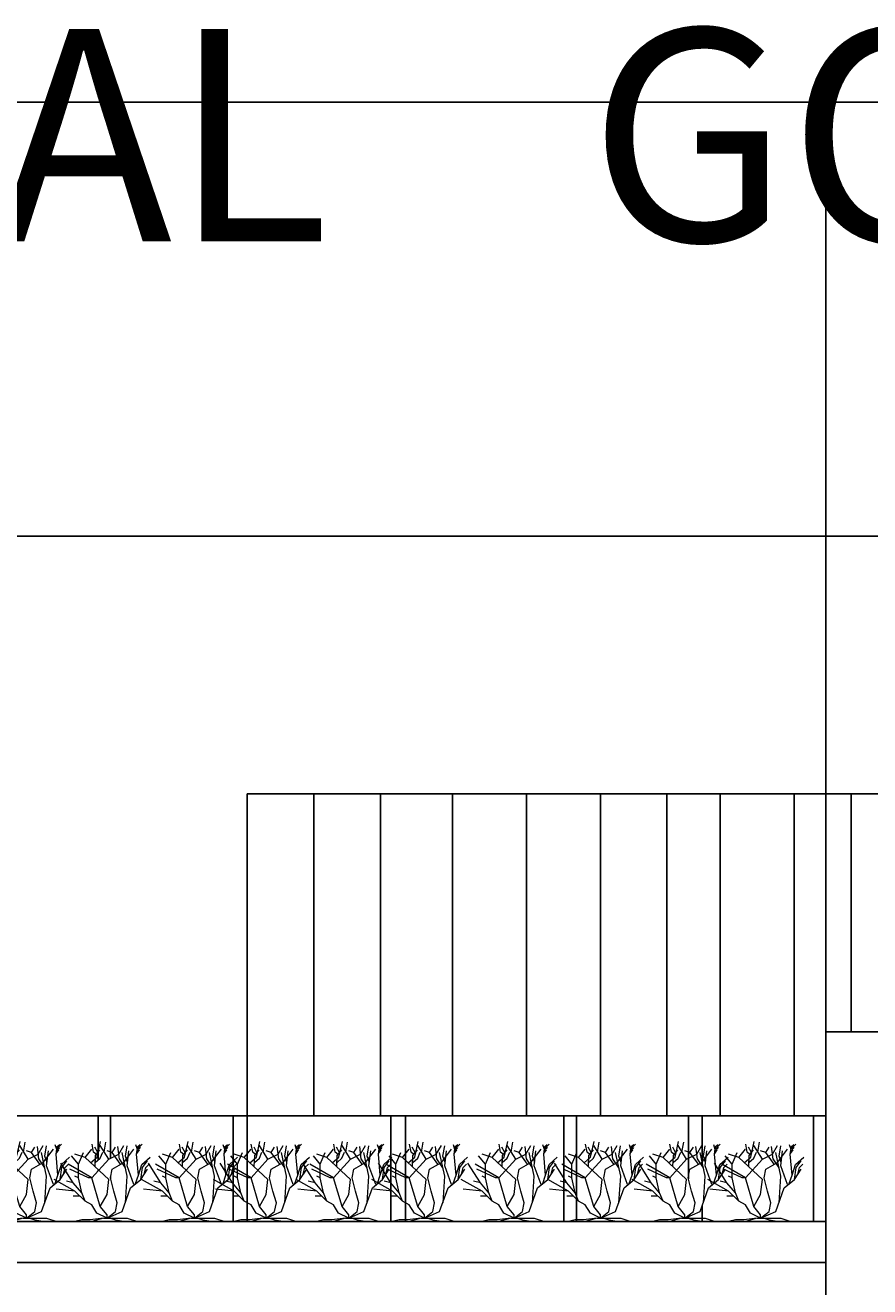
# Model space of a CAD drawing. Units: inches. Extents: x -117 to 121, y -77 to 40.
# Tile 17 of 45: x -45 to -23, y 7 to 40. Entities that reach past the tile are written whole.
import ezdxf

# ---------------------------------------------------------------- set-up
doc = ezdxf.new("R2010")
doc.units = ezdxf.units.IN
doc.header["$MEASUREMENT"] = 0
for name, color, linetype, lineweight in [('A-ANNO-DIMS', 2, 'Continuous', 18), ('A-ANNO-TEXT', 7, 'Continuous', 25), ('A-ELEV', 7, 'Continuous', 25), ('L-PLNT', 3, 'Continuous', 13)]:
    doc.layers.add(name, color=color, linetype=linetype, lineweight=lineweight)
doc.styles.get("Standard").update_dxf_attribs({"font": 'arial.ttf'})
doc.dimstyles.get("Standard").update_dxf_attribs({"dimtxt": 0.18, "dimasz": 0.18, "dimexe": 0.18, "dimexo": 0.0625, "dimgap": 0.09, "dimtad": 0, "dimtih": 1, "dimtoh": 1, "dimdec": 4, "dimzin": 0, "dimdsep": 46, "dimtxsty": 'Standard', "dimcen": 0.09, "dimadec": 0, "dimazin": 0, "dimtfac": 1, "dimtdec": 4, "dimtofl": 0, "dimtmove": 0, "dimatfit": 3, "dimfxl": 1, "dimtolj": 1, "dimtzin": 0, "dimarcsym": 0})

# ---------------------------------------------------------------- blocks, each defined once
blk = doc.blocks.new('*U3')
for p, q in [((-12.471, 19.775), (-12.898, 22.044)), ((-11.433, 18.289), (-10.457, 22.749)), ((-8.16, 17.76), (-10.56, 21.6)), ((-9.48, 19.775), (-8.992, 22.592)), ((-5.28, 19.2), (-3.84, 21.6)), ((-3.377, 18.602), (-2.888, 21.575)), ((-0.508, 21.888), (-0.081, 20.558)), ((0.041, 20.714), (1.384, 22.044)), ((0.102, 21.34), (0.835, 21.888)), ((-16.8, 16.32), (-18.72, 18.72)), ((-14.88, 18.24), (-17.76, 19.2)), ((-16.8, 16.32), (-15.36, 19.68)), ((-14.88, 18.24), (-12.96, 20.64)), ((-8.16, 12), (-14.88, 18.24)), ((-13.325, 16.724), (-11.433, 18.289)), ((-11.677, 19.071), (-12.471, 19.775)), ((-11.28, 19.619), (-12.104, 21.184)), ((-12.043, 15.628), (-11.921, 18.836)), ((-11.982, 16.802), (-10.579, 18.054)), ((-11.921, 18.836), (-10.64, 20.401)), ((-10.579, 18.054), (-9.846, 19.697)), ((-7.2, 19.68), (-8.64, 20.16)), ((-8.16, 17.76), (-5.28, 19.2)), ((-7.2, 19.68), (-6.24, 21.12)), ((-4.8, 16.32), (-7.2, 19.68)), ((-5.086, 17.741), (-5.513, 21.34)), ((-2.88, 12.96), (-4.32, 19.68)), ((-3.84, 16.8), (-0.96, 20.64)), ((-2.766, 16.802), (-3.377, 18.602)), ((-2.88, 15.84), (-2.4, 20.16)), ((-0.203, 19.149), (0.102, 21.34)), ((0.346, 13.203), (-0.203, 19.149)), ((-0.142, 19.384), (0.59, 20.401)), ((-0.02, 20.01), (0.896, 21.105)), ((1.323, 16.254), (3.642, 18.289)), ((-18.24, 11.04), (-21.755, 16.655)), ((-12.96, 12.48), (-19.68, 16.32)), ((-13.92, 12.48), (-19.2, 14.88)), ((-16.8, 12.48), (-16.8, 16.32)), ((-12.96, 12.48), (-8.16, 17.76)), ((-7.68, 12.48), (-7.2, 14.88)), ((-7.2, 14.88), (-3.84, 16.8)), ((-3.377, 15.315), (-5.086, 17.819)), ((-0.96, 10.56), (-2.88, 15.84)), ((0.346, 13.203), (1.323, 16.254)), ((0.96, 12), (1.44, 15.36)), ((0.96, 12), (2.88, 14.88)), ((1.44, 15.36), (2.88, 17.28)), ((1.92, 13.44), (2.4, 15.36)), ((2.4, 15.36), (3.36, 16.32)), ((-17.76, 8.64), (-23.663, 11.961)), ((-18.24, 11.04), (-20.16, 11.52)), ((-15.84, 8.16), (-18.24, 11.04)), ((-16.8, 12.48), (-17.76, 12.96)), ((-15.84, 8.16), (-16.8, 12.48)), ((-12.96, 12.48), (-13.92, 12.48)), ((-10.56, 4.32), (-12.96, 12.48)), ((-8.64, 7.68), (-8.16, 12)), ((-6.72, 8.64), (-7.68, 12.48)), ((-3.36, 5.28), (-2.88, 12.96)), ((-1.92, 9.6), (0.96, 12)), ((-0.48, 10.8), (0.346, 13.203)), ((-17.76, 8.64), (-23.128, 9.222)), ((-16.32, 7.2), (-18.24, 7.2)), ((-14.88, 5.76), (-17.76, 8.64)), ((-14.88, 5.76), (-15.84, 8.16)), ((-10.56, 4.32), (-8.64, 7.68)), ((-5.76, 5.28), (-6.72, 8.64)), ((-4.32, 2.88), (-1.92, 9.6)), ((-12.96, 4.8), (-14.88, 5.76)), ((-11.52, 2.4), (-12.96, 4.8)), ((-8.64, 1.92), (-10.56, 4.32)), ((-6.24, 2.88), (-5.76, 5.28)), ((-15.84, 0.48), (-17.76, 0)), ((-13.44, 0.48), (-15.84, 0.48)), ((-9.6, 0.96), (-13.44, 0.48)), ((-9.6, 0.96), (-12.96, 0)), ((-8.64, 0.96), (-11.52, 2.4)), ((-9.6, 0.96), (-7.68, 0.96)), ((-8.64, 0.96), (-4.32, 2.88)), ((-8.64, 0.96), (-6.24, 2.88)), ((-8.64, 0.96), (-8.64, 1.92)), ((-8.64, 0.96), (-2.88, 0.96)), ((-7.68, 0.96), (-6.24, 0.48)), ((-6.24, 0.48), (-3.36, 0)), ((-2.88, 0.96), (0, 0))]:
    blk.add_line(p, q)
blk = doc.blocks.new('*D9')
at = {"layer": 'A-ANNO-DIMS', "color": 0, "lineweight": -2, "transparency": 16777216}
for p, q in [((-75.804, 8.087), (-75.804, 38.61)), ((-75.624, 38.43), (-50.227, 38.43)), ((-24.044, 38.43), (-49.44, 38.43)), ((-23.864, 8.087), (-23.864, 38.61))]:
    blk.add_line(p, q, dxfattribs=at)
at = {"layer": 'A-ANNO-DIMS', "color": 0, "transparency": 16777216}
for points in [[(-75.624, 38.46), (-75.624, 38.4), (-75.804, 38.43)], [(-24.044, 38.46), (-24.044, 38.4), (-23.864, 38.43)]]:
    blk.add_solid(points, dxfattribs=at)
at = {"layer": 'Defpoints', "color": 0, "transparency": 16777216}
for p in [(-23.864, 38.43), (-75.804, 8.025), (-23.864, 8.025)]:
    blk.add_point(p, dxfattribs=at)
at = {"layer": 'A-ANNO-DIMS', "color": 0, "transparency": 16777216, "insert": (-49.834, 38.43), "char_height": 0.18, "attachment_point": 5}
blk.add_mtext('\\A1;51.94', dxfattribs=at)
blk = doc.blocks.new('*D13')
at = {"layer": 'A-ANNO-DIMS', "color": 0, "lineweight": -2, "transparency": 16777216}
for p, q in [((-2.663, 27.063), (-117.024, 27.063)), ((-116.844, 26.883), (-116.844, -16.974)), ((-116.844, -61.196), (-116.844, -17.338)), ((-106.096, -61.376), (-117.024, -61.376))]:
    blk.add_line(p, q, dxfattribs=at)
at = {"layer": 'A-ANNO-DIMS', "color": 0, "transparency": 16777216}
for points in [[(-116.874, 26.883), (-116.814, 26.883), (-116.844, 27.063)], [(-116.874, -61.196), (-116.814, -61.196), (-116.844, -61.376)]]:
    blk.add_solid(points, dxfattribs=at)
at = {"layer": 'Defpoints', "color": 0, "transparency": 16777216}
for p in [(-2.6, 27.063), (-116.844, -61.376), (-106.034, -61.376)]:
    blk.add_point(p, dxfattribs=at)
at = {"layer": 'A-ANNO-DIMS', "color": 0, "transparency": 16777216, "insert": (-116.844, -17.156), "char_height": 0.18, "attachment_point": 5}
blk.add_mtext('\\A1;88.44', dxfattribs=at)
blk = doc.blocks.new('*D22')
at = {"layer": 'A-ANNO-DIMS', "color": 0, "lineweight": -2, "transparency": 16777216}
for p, q in [((-23.864, 8.087), (-23.864, 38.61)), ((-23.684, 38.43), (-13.697, 38.43)), ((-2.78, 38.43), (-12.767, 38.43)), ((-2.6, 27.126), (-2.6, 38.61))]:
    blk.add_line(p, q, dxfattribs=at)
at = {"layer": 'A-ANNO-DIMS', "color": 0, "transparency": 16777216}
for points in [[(-23.684, 38.46), (-23.684, 38.4), (-23.864, 38.43)], [(-2.78, 38.46), (-2.78, 38.4), (-2.6, 38.43)]]:
    blk.add_solid(points, dxfattribs=at)
at = {"layer": 'Defpoints', "color": 0, "transparency": 16777216}
for p in [(-2.6, 38.43), (-2.6, 27.063), (-23.864, 8.025)]:
    blk.add_point(p, dxfattribs=at)
at = {"layer": 'A-ANNO-DIMS', "color": 0, "transparency": 16777216, "insert": (-13.232, 38.43), "char_height": 0.18, "attachment_point": 5}
blk.add_mtext('\\A1;21.264', dxfattribs=at)

msp = doc.modelspace()

# ---------------------------------------------------------------- linework, layer by layer
at = {"layer": 'A-ELEV'}
for p, q in [((-21.1993, 20.3104), (-39.0355, 20.3104)), ((-39.0355, 20.3104), (-39.0355, 9.0994)), ((-37.2854, 11.8711), (-37.2854, 20.3104)), ((-35.5436, 11.8711), (-35.5436, 20.3104)), ((-33.6526, 11.8711), (-33.6526, 20.3104)), ((-31.7118, 11.8711), (-31.7118, 20.3104)), ((-29.7709, 11.8711), (-29.7709, 20.3104)), ((-28.0292, 11.8711), (-28.0292, 20.3104)), ((-26.6358, 11.8711), (-26.6358, 20.3104)), ((-24.6949, 11.8711), (-24.6949, 20.3104)), ((-23.202, 14.0735), (-23.202, 20.3104)), ((-23.8637, 14.0735), (-23.8637, 2.5407)), ((-21.1993, 14.0735), (-23.8637, 14.0735)), ((-75.8037, 11.8711), (-23.8637, 11.8711)), ((-42.9411, 10.7156), (-42.9411, 11.8711)), ((-42.6199, 10.7574), (-42.6199, 11.8711)), ((-39.4048, 9.0994), (-39.4048, 11.8711)), ((-35.2711, 9.0994), (-35.2711, 11.8711)), ((-34.8856, 9.0994), (-34.8856, 11.8711)), ((-30.7356, 9.0994), (-30.7356, 11.8711)), ((-30.4002, 9.0994), (-30.4002, 11.8711)), ((-27.4631, 10.2178), (-27.4631, 11.8711)), ((-27.1047, 10.5528), (-27.1047, 11.8711)), ((-24.1906, 9.0994), (-24.1906, 11.8711)), ((-42.9411, 10.4332), (-42.9411, 10.4559)), ((-42.6199, 10.2296), (-42.6199, 10.2686)), ((-42.6199, 9.2275), (-42.6199, 9.2605)), ((-27.4631, 9.1839), (-27.4631, 9.2628)), ((-27.1047, 9.0994), (-27.1047, 9.5206)), ((-23.8637, 9.0994), (-75.8037, 9.0994)), ((-42.9411, 9.1463), (-42.9411, 9.1688)), ((-42.6199, 9.1848), (-42.6199, 9.1863)), ((-23.8637, 8.0246), (-75.8037, 8.0246))]:
    msp.add_line(p, q, dxfattribs=at)

# ---------------------------------------------------------------- block references
at = {"layer": 'L-PLNT', "xscale": 0.0920717077623056, "yscale": 0.0920717077623056, "zscale": 0.0920717077623056}
for p in [(-44.0301, 9.0979), (-41.9171, 9.0979), (-39.6259, 9.0979), (-37.742, 9.0979), (-35.5781, 9.0979), (-33.5923, 9.0979), (-31.2439, 9.0979), (-28.9781, 9.0979), (-26.7633, 9.0979), (-24.7775, 9.0979)]:
    msp.add_blockref('*U3', p, dxfattribs=at)

# ---------------------------------------------------------------- texts
at = {"layer": 'A-ANNO-TEXT'}
msp.add_text('CONCEPTUAL    GOOD   VIBE   CAFE   DESIGN', height=5.56486, dxfattribs=at).set_placement((-85.726, 34.7863))

# ---------------------------------------------------------------- dimensions: what is measured, and where the dimension line sits
at = {"layer": 'A-ANNO-DIMS'}
for base, p1, p2, override, picture, middle in [((-23.8637, 38.4297), (-75.8037, 8.0246), (-23.8637, 8.0246), {"dimdec": 2, "dimlfac": 1, "dimrnd": 0, "dimzin": 0, "dimdsep": 46, "dimlunit": 2}, '*D9', (-49.8337, 38.4297)), ((-2.6001, 38.4297), (-23.8637, 8.0246), (-2.6001, 27.0634), {"dimdec": 3, "dimlfac": 1, "dimrnd": 0, "dimzin": 0, "dimdsep": 46, "dimlunit": 2}, '*D22', (-13.2319, 38.4297))]:
    dim = msp.add_linear_dim(base=base, p1=p1, p2=p2, dimstyle='Standard', override=override, dxfattribs=at)
    dim.commit()
    dim.dimension.update_dxf_attribs({"geometry": picture, "text_midpoint": middle})
dim = msp.add_linear_dim(base=(-116.8438, -61.3756), p1=(-2.6001, 27.0634), p2=(-106.0338, -61.3756), angle=90, dimstyle='Standard', override={"dimdec": 2, "dimlfac": 1, "dimrnd": 0, "dimzin": 0, "dimdsep": 46, "dimlunit": 2}, dxfattribs=at)
dim.commit()
dim.dimension.update_dxf_attribs({"geometry": '*D13', "text_midpoint": (-116.8438, -17.1561)})

doc.saveas('drawing.dxf')
